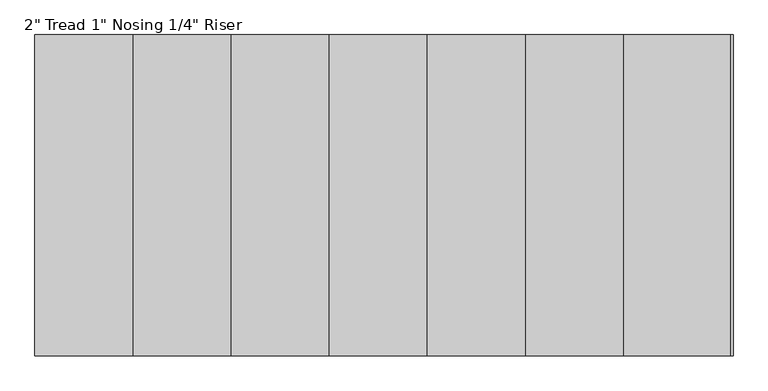
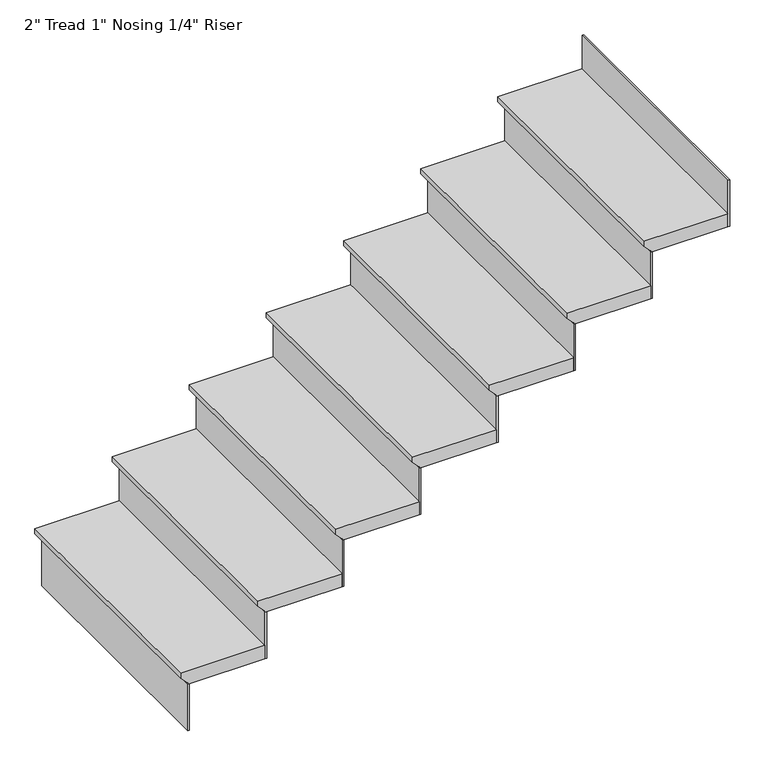
"""IFC4 building model written with IfcOpenShell, lengths in millimetres: stair flight geometry."""

from ifc_helpers import new_model, si_unit, frame, origin, place, context, project, spatial, polyline, outline, extrude, source, transform, mapped, element, save


def stair_flight_13cb1edf(model_context):
    return source(origin(), model_context, "Body", "SweptSolid", [
        extrude(outline(polyline([(12166.6, -11753.6120641), (12166.6, -12058.4120641), (12147.55, -12058.4120641), (12122.15, -12033.0120641), (12115.8, -12033.0120641), (12115.8, -11753.6120641), (12166.6, -11753.6120641)])), frame((0.0, -4817.9038196, 0.0), z_axis=(0.0, 1.0, 0.0), x_axis=(0.0, 0.0, 1.0)), (0.0, 0.0, 1.0), 914.4),
        extrude(outline(polyline([(-12026.6620641, -4817.9038196), (-12033.0120641, -4817.9038196), (-12033.0120641, -3903.5038196), (-12026.6620641, -3903.5038196), (-12026.6620641, -4817.9038196)])), frame((0.0, 0.0, 11938.0), z_axis=(0.0, 0.0, 1.0), x_axis=(1.0, 0.0, 0.0)), (0.0, 0.0, 1.0), 177.8),
        extrude(outline(polyline([(-11747.2620641, -4817.9038196), (-11753.6120641, -4817.9038196), (-11753.6120641, -3903.5038196), (-11747.2620641, -3903.5038196), (-11747.2620641, -4817.9038196)])), frame((0.0, 0.0, 12115.8), z_axis=(0.0, 0.0, 1.0), x_axis=(1.0, 0.0, 0.0)), (0.0, 0.0, 1.0), 177.8),
        extrude(outline(polyline([(12344.4, -11474.2120641), (12344.4, -11779.0120641), (12325.35, -11779.0120641), (12299.95, -11753.6120641), (12293.6, -11753.6120641), (12293.6, -11474.2120641), (12344.4, -11474.2120641)])), frame((0.0, -4817.9038196, 0.0), z_axis=(0.0, 1.0, 0.0), x_axis=(0.0, 0.0, 1.0)), (0.0, 0.0, 1.0), 914.4),
        extrude(outline(polyline([(-11467.8620641, -4817.9038196), (-11474.2120641, -4817.9038196), (-11474.2120641, -3903.5038196), (-11467.8620641, -3903.5038196), (-11467.8620641, -4817.9038196)])), frame((0.0, 0.0, 12293.6), z_axis=(0.0, 0.0, 1.0), x_axis=(1.0, 0.0, 0.0)), (0.0, 0.0, 1.0), 177.8),
        extrude(outline(polyline([(12522.2, -11194.8120641), (12522.2, -11499.6120641), (12503.15, -11499.6120641), (12477.75, -11474.2120641), (12471.4, -11474.2120641), (12471.4, -11194.8120641), (12522.2, -11194.8120641)])), frame((0.0, -4817.9038196, 0.0), z_axis=(0.0, 1.0, 0.0), x_axis=(0.0, 0.0, 1.0)), (0.0, 0.0, 1.0), 914.4),
        extrude(outline(polyline([(-11188.4620641, -4817.9038196), (-11194.8120641, -4817.9038196), (-11194.8120641, -3903.5038196), (-11188.4620641, -3903.5038196), (-11188.4620641, -4817.9038196)])), frame((0.0, 0.0, 12471.4), z_axis=(0.0, 0.0, 1.0), x_axis=(1.0, 0.0, 0.0)), (0.0, 0.0, 1.0), 177.8),
        extrude(outline(polyline([(12700.0, -10915.4120641), (12700.0, -11220.2120641), (12680.95, -11220.2120641), (12655.55, -11194.8120641), (12649.2, -11194.8120641), (12649.2, -10915.4120641), (12700.0, -10915.4120641)])), frame((0.0, -4817.9038196, 0.0), z_axis=(0.0, 1.0, 0.0), x_axis=(0.0, 0.0, 1.0)), (0.0, 0.0, 1.0), 914.4),
        extrude(outline(polyline([(-10909.0620641, -4817.9038196), (-10915.4120641, -4817.9038196), (-10915.4120641, -3903.5038196), (-10909.0620641, -3903.5038196), (-10909.0620641, -4817.9038196)])), frame((0.0, 0.0, 12649.2), z_axis=(0.0, 0.0, 1.0), x_axis=(1.0, 0.0, 0.0)), (0.0, 0.0, 1.0), 177.8),
        extrude(outline(polyline([(12877.8, -10636.0120641), (12877.8, -10940.8120641), (12858.75, -10940.8120641), (12833.35, -10915.4120641), (12827.0, -10915.4120641), (12827.0, -10636.0120641), (12877.8, -10636.0120641)])), frame((0.0, -4817.9038196, 0.0), z_axis=(0.0, 1.0, 0.0), x_axis=(0.0, 0.0, 1.0)), (0.0, 0.0, 1.0), 914.4),
        extrude(outline(polyline([(-10629.6620641, -4817.9038196), (-10636.0120641, -4817.9038196), (-10636.0120641, -3903.5038196), (-10629.6620641, -3903.5038196), (-10629.6620641, -4817.9038196)])), frame((0.0, 0.0, 12827.0), z_axis=(0.0, 0.0, 1.0), x_axis=(1.0, 0.0, 0.0)), (0.0, 0.0, 1.0), 177.8),
        extrude(outline(polyline([(13055.6, -10356.6120641), (13055.6, -10661.4120641), (13036.55, -10661.4120641), (13011.15, -10636.0120641), (13004.8, -10636.0120641), (13004.8, -10356.6120641), (13055.6, -10356.6120641)])), frame((0.0, -4817.9038196, 0.0), z_axis=(0.0, 1.0, 0.0), x_axis=(0.0, 0.0, 1.0)), (0.0, 0.0, 1.0), 914.4),
        extrude(outline(polyline([(-10350.2620641, -4817.9038196), (-10356.6120641, -4817.9038196), (-10356.6120641, -3903.5038196), (-10350.2620641, -3903.5038196), (-10350.2620641, -4817.9038196)])), frame((0.0, 0.0, 13004.8), z_axis=(0.0, 0.0, 1.0), x_axis=(1.0, 0.0, 0.0)), (0.0, 0.0, 1.0), 177.8),
        extrude(outline(polyline([(-10070.8620641, -4817.9038196), (-10077.2120641, -4817.9038196), (-10077.2120641, -3903.5038196), (-10070.8620641, -3903.5038196), (-10070.8620641, -4817.9038196)])), frame((0.0, 0.0, 13182.6), z_axis=(0.0, 0.0, 1.0), x_axis=(1.0, 0.0, 0.0)), (0.0, 0.0, 1.0), 177.8),
        extrude(outline(polyline([(13233.4, -10077.2120641), (13233.4, -10382.0120641), (13214.35, -10382.0120641), (13188.95, -10356.6120641), (13182.6, -10356.6120641), (13182.6, -10077.2120641), (13233.4, -10077.2120641)])), frame((0.0, -4817.9038196, 0.0), z_axis=(0.0, 1.0, 0.0), x_axis=(0.0, 0.0, 1.0)), (0.0, 0.0, 1.0), 914.4),
    ])


if __name__ == "__main__":
    model = new_model("IFC4")
    model_context = context("Model", 3, world=origin())
    ifc_project = project(units=[si_unit("LENGTHUNIT", "METRE", prefix="MILLI")], contexts=[model_context])
    site = spatial("IfcSite", under=ifc_project)
    building = spatial("IfcBuilding", under=site)
    placement = place(None, origin())
    stair_flight_shape = stair_flight_13cb1edf(model_context)
    element("IfcStairFlight", 1, ObjectType="2\" Tread 1\" Nosing 1/4\" Riser", at=placement, inside=building, context=model_context, shape_type="MappedRepresentation", body=[
        mapped(stair_flight_shape, transform((0.0, 0.0, 0.0), x_axis=(1.0, 0.0, 0.0), y_axis=(0.0, 1.0, 0.0), z_axis=(0.0, 0.0, 1.0))),
    ])
    save(model, "model.ifc")
